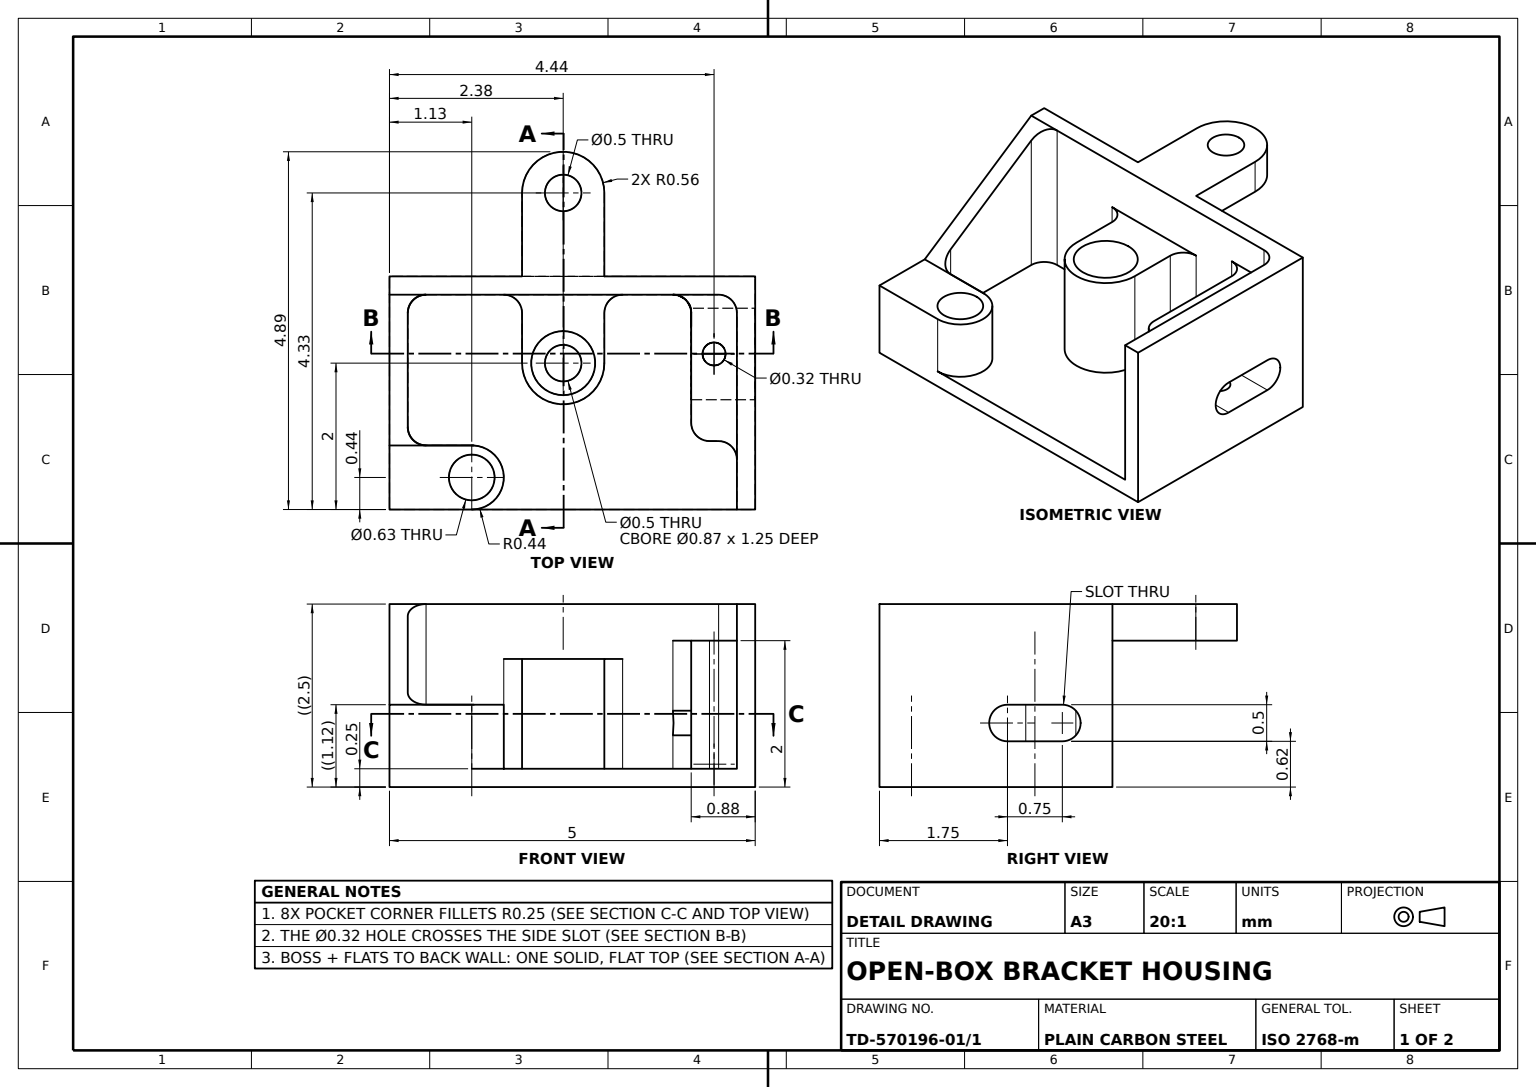
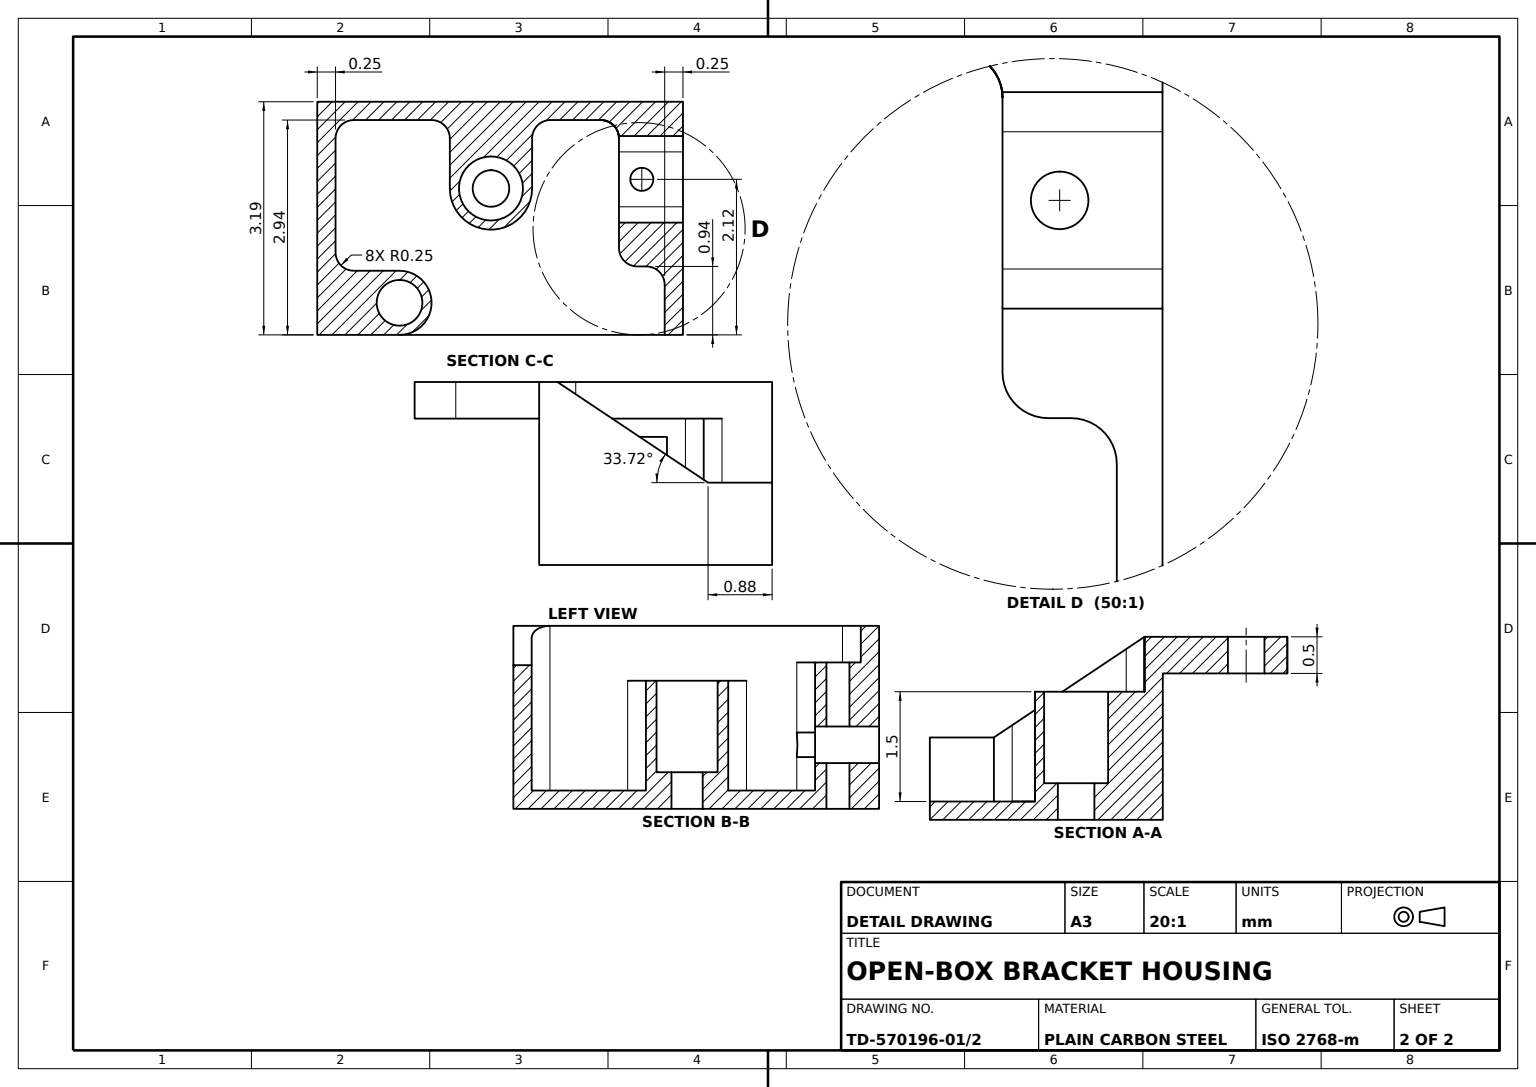
SolidWorks part; units mm, degrees
material "Plain Carbon Steel"
ref_plane "Front Plane" through (0, 0, 0) normal (0, 0, 1) x (1, 0, 0)
ref_plane "Top Plane" through (0, 0, 0) normal (0, 1, 0) x (1, 0, 0)
ref_plane "Right Plane" through (0, 0, 0) normal (1, 0, 0) x (0, 0, -1)
sketch "Base Plate Sketch" plane through (0, 0, 0) normal (0, 1, 0) x (1, 0, 0)
  line L0 (0, 0) -> (2.5, 0)
  line L1 (2.5, 0) -> (2.5, 3.185)
  line L2 (2.5, 3.185) -> (-2.5, 3.185)
  line L3 (-2.5, 3.185) -> (-2.5, 0)
  line L4 (-2.5, 0) -> (0, 0)
  dimension "D1" = 5
  dimension "D2" = 3.185
  dimension "D3" = 2.5
extrude "Base Plate" add sketch "Base Plate Sketch" along normal blind 0.25
sketch "Perimeter Walls Sketch" plane through (0, 0.25, 0) normal (0, 1, 0) x (1, 0, 0)
  line L0 (-2.5, 0) -> (-2.5, 3.185)
  line L1 (-2.5, 3.185) -> (2.5, 3.185)
  line L2 (2.5, 3.185) -> (2.5, 0)
  line L3 (-2.25, 0) -> (-2.25, 2.935)
  line L4 (-2.25, 2.935) -> (2.25, 2.935)
  line L5 (2.25, 2.935) -> (2.25, 0)
  line L6 (-2.5, 0) -> (-2.25, 0)
  line L7 (2.25, 0) -> (2.5, 0)
  dimension "D1" = 0.25
extrude "Perimeter Walls" add sketch "Perimeter Walls Sketch" along normal blind 2.25
sketch "Corner Boss Sketch" plane through (0, 0.25, 0) normal (0, 1, 0) x (1, 0, 0)
  line L0 (-2.5, 0) -> (-2.5, 0.438)
  line L1 (-2.5, 3.185) -> (-2.5, 0) construction
  line L3 (-1.375, 0) -> (-2.5, 0)
  line L4 (-1.375, 0.876) -> (-2.5, 0.876)
  line L5 (-2.5, 0.876) -> (-2.5, 0.438)
  arc A0 (-1.375, 0) -> (-1.375, 0.876) centre (-1.375, 0.438) ccw
  dimension "D1" = 0.438
  dimension "D2" = 1.375
  dimension "D3" = 0.438
extrude "Corner Boss" add sketch "Corner Boss Sketch" along normal blind 1.125
sketch "Wall Pocket Sketch" plane through (-2.5, 0, 0) normal (-1, 0, 0) x (0, 0, 1)
  line L0 (0, 2.5) -> (-2.935, 2.5)
  line L1 (-3.185, 2.5) -> (0, 2.5) construction
  line L2 (-3.185, 0) -> (0, 0) construction
  line L3 (0, 2.5) -> (0, 0) construction
  line L4 (0, 1.125) -> (-0.875, 1.125)
  line L5 (-0.875, 1.125) -> (-2.935, 2.5)
  line L6 (0, 2.5) -> (0, 1.125)
  dimension "D1" = 0.875
  dimension "D2" = 2.935
  dimension "D3" = 1.125
extrude "Wall Pocket Cut" cut sketch "Wall Pocket Sketch" against normal blind 2.125
sketch "Central Boss Sketch" plane through (0, 0.25, 0) normal (0, 1, 0) x (1, 0, 0)
  line L0 (-2.5, 0) -> (-0.125, 0)
  line L1 (-1.375, 0) -> (2.25, 0) construction
  line L3 (0.4375, 2) -> (0.4375, 2.935)
  line L4 (-2.25, 2.935) -> (2.25, 2.935) construction
  line L5 (-0.6875, 2) -> (-0.6875, 3.185)
  line L6 (2.5, 3.185) -> (-2.5, 3.185) construction
  line L7 (-0.6875, 3.185) -> (0.4375, 3.185)
  line L8 (0.4375, 3.185) -> (0.4375, 2.935)
  arc A0 (-0.6875, 2) -> (0.4375, 2) centre (-0.125, 2) ccw
  line M5 (2.25, 2.935) -> (-2.25, 2.935)
  dimension "D1" = 0.5625
  dimension "D2" = 0.125
  dimension "D3" = 2.0039
extrude "Central Boss" add sketch "Central Boss Sketch" along normal blind 1.5 contours L5 A0 L3 M5
sketch "Mounting Tab Sketch" plane through (0, 0.25, 0) normal (0, 1, 0) x (1, 0, 0)
  line L0 (2.5, 3.185) -> (2.5, 0.935)
  line L1 (2.5, 0) -> (2.5, 3.185) construction
  line L2 (2.5, 0.935) -> (1.625, 0.935)
  line L3 (1.625, 0.935) -> (1.625, 2.935)
  line L4 (-2.25, 2.935) -> (2.25, 2.935) construction
  line L5 (1.625, 2.935) -> (1.625, 3.185)
  line L8 (2.5, 3.185) -> (-2.5, 3.185) construction
  line L9 (1.625, 3.185) -> (2.5, 3.185)
  dimension "D1" = 2
  dimension "D2" = 0.875
extrude "Mounting Tab" add sketch "Mounting Tab Sketch" along normal blind 1.75
sketch "Side Slot Sketch" plane through (2.5, 0, 0) normal (1, 0, 0) x (0, 0, -1)
  line L4 (1.75, 1.125) -> (2.5, 1.125)
  line L5 (1.75, 0.625) -> (2.5, 0.625)
  arc A0 (1.75, 1.125) -> (1.75, 0.625) centre (1.75, 0.875) ccw
  arc A1 (2.5, 0.625) -> (2.5, 1.125) centre (2.5, 0.875) ccw
  dimension "D1" = 0.5
  dimension "D2" = 1.75
  dimension "D3" = 0.875
  dimension "D4" = 0.75
extrude "Side Wall Slot" cut sketch "Side Slot Sketch" against normal blind 1.75
sketch "Wall Lip Sketch" plane through (0, 2.5, 0) normal (0, 1, 0) x (1, 0, 0)
  line L0 (-0.6875, 2.935) -> (0.4375, 2.935)
  line L1 (0.4375, 4.325) -> (0.4375, 2.935)
  line L2 (-0.6875, 4.325) -> (-0.6875, 2.935)
  arc A0 (0.4375, 4.325) -> (-0.6875, 4.325) centre (-0.125, 4.325) ccw
  dimension "D1" = 4.325
extrude "Wall Lip" add sketch "Wall Lip Sketch" against normal blind 0.5
sketch "Profile Trim Sketch" plane through (0, 2.5, 0) normal (0, 1, 0) x (1, 0, 0)
  circle A0 centre (-0.125, 4.325) radius 0.25
  circle A1 centre (1.9375, 2.125) radius 0.1575
  circle A2 centre (-1.375, 0.438) radius 0.2205
  circle A3 centre (-0.125, 2) radius 0.25
  dimension "D1" = 0.5
  dimension "D2" = 0.315
  dimension "D3" = 0.5
  dimension "D4" = 0.441
  dimension "D5" = 1.9375
  dimension "D6" = 2.125
extrude "Profile Trim Cut" cut sketch "Profile Trim Sketch" against normal blind 3.5
fillet "Tab Edge Fillet R0.25" radius 0.25 1 edges at (1.625, 1.125, -0.935)
fillet "Tab-Wall Fillet 1 R0.25" radius 0.25 1 edges at (2.25, 1.125, -0.935)
fillet "Tab-Wall Fillet 2 R0.25" radius 0.25 1 edges at (1.625, 1.125, -2.935)
fillet "Central Boss Fillet 1 R0.25" radius 0.25 1 edges at (0.4375, 1, -2.935)
fillet "Central Boss Fillet 2 R0.25" radius 0.25 1 edges at (-0.6875, 1, -2.935)
fillet "Wall Fillet 1 R0.25" radius 0.25 1 edges at (-2.25, 1.375, -2.935)
fillet "Corner Boss Fillet R0.25" radius 0.25 1 edges at (-2.25, 0.6878, -0.876)
fillet "Wall Fillet 2 R0.25" radius 0.25 1 edges at (2.25, 2.25, -2.935)
sketch "Boss Hole Sketch Ø0.875" plane through (0, 1.75, 0) normal (0, 1, 0) x (1, 0, 0)
  circle A0 centre (-0.125, 2) radius 0.4375
  dimension "D1" = 0.875
extrude "Boss Hole Ø0.875" cut sketch "Boss Hole Sketch Ø0.875" against normal blind 1.25
sketch "Hole Sketch Ø0.625" plane through (0, 1.125, 0) normal (0, 1, 0) x (1, 0, 0)
  circle A0 centre (-1.375, 0.438) radius 0.3125
  dimension "D1" = 0.625
extrude "Hole Ø0.625" cut sketch "Hole Sketch Ø0.625" against normal blind 1.25
